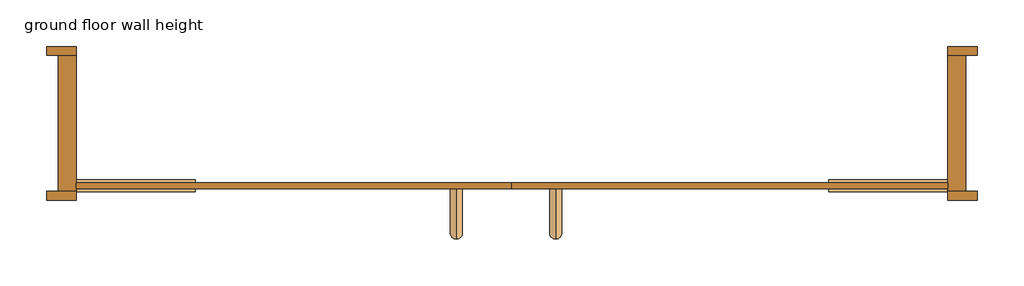
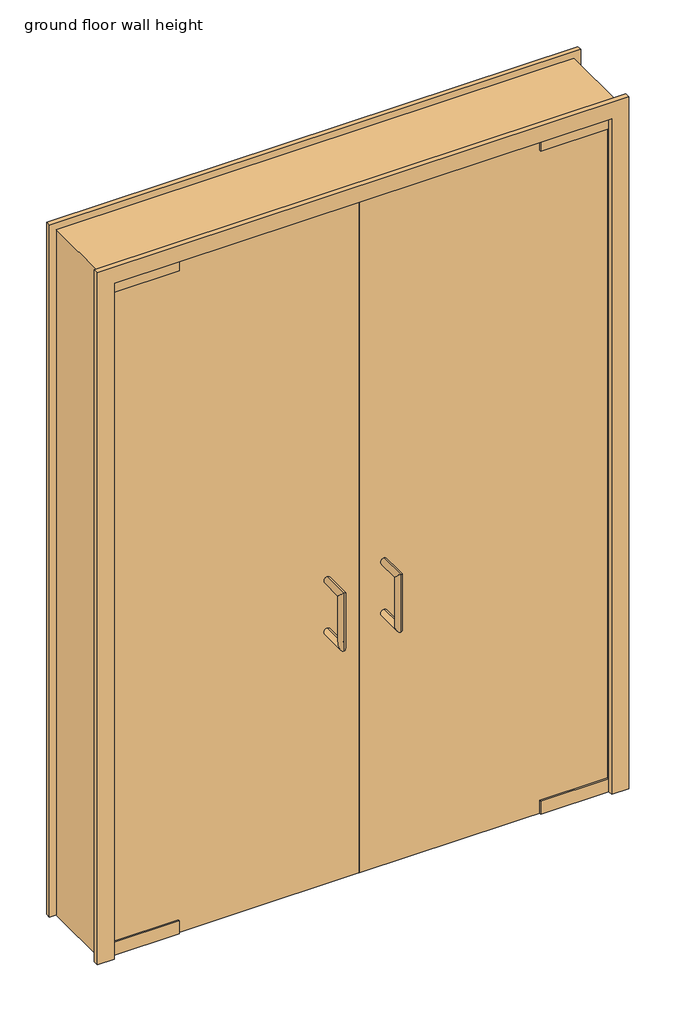
# One storey: 1 door.
"""IFC4 building model written with IfcOpenShell, lengths in millimetres."""

from ifc_helpers import new_model, si_unit, origin, place, context, project, spatial, transform, mapped, element, save
from components import double_metal_frame_w_glass_1524_x_2134_5eb37b3f

model = new_model("IFC4")

# Units and contexts
model_context = context("Model", 3, world=origin())
ifc_project = project(units=[si_unit("LENGTHUNIT", "METRE", prefix="MILLI")], contexts=[model_context])

# Site, building, storey
site = spatial("IfcSite", under=ifc_project)
building = spatial("IfcBuilding", under=site)
storey = spatial("IfcBuildingStorey", under=building, Name="ground floor wall height", Elevation=3048.0)

# Door
placement = place(None, origin())
double_metal_frame_w_glass_1524_x_2134_shape = double_metal_frame_w_glass_1524_x_2134_5eb37b3f(model_context)
element("IfcDoor", 1, ObjectType="Double-Metal Frame w Glass : 1524 x 2134", at=placement, inside=storey, context=model_context, shape_type="MappedRepresentation", body=[
    mapped(double_metal_frame_w_glass_1524_x_2134_shape, transform((-5858.4678816, 2726.2030358, 3048.0), x_axis=(-1.0, 0.0, 0.0), y_axis=(0.0, -1.0, 0.0), z_axis=(0.0, 0.0, 1.0))),
])

save(model, "model.ifc")

# Revit data of these elements
# Type "Double-Metal Frame w Glass : 1524 x 2134"
#   Type Mark = "17"
#   Operation = "DoubleDoorSingleSwing"
#   Keynote = "L20"
#   Analytic Construction = "<None>"
#   Height = 7' - 0"
#   Width = 5' - 0"
#   Define Thermal Properties by = 1
#   Wall Closure = (empty or 0)
#   Function = (empty or 0)
# Element 1 (IfcDoor, "Double-Metal Frame w Glass : 1524 x 2134")
#   Phase Created = New Construction
#   Materials on its faces: "Chrome", "Default Metal Frame", "Glass"
# Materials
#   "Chrome": colour RGB 192 192 192, transparency 0
#   "Default Metal Frame": colour RGB 132 153 165, transparency 0
#   "Glass": class "Glass", colour RGB 0 128 192, transparency 0.75, Description = "Soda Lime Glass", Cost = 0
